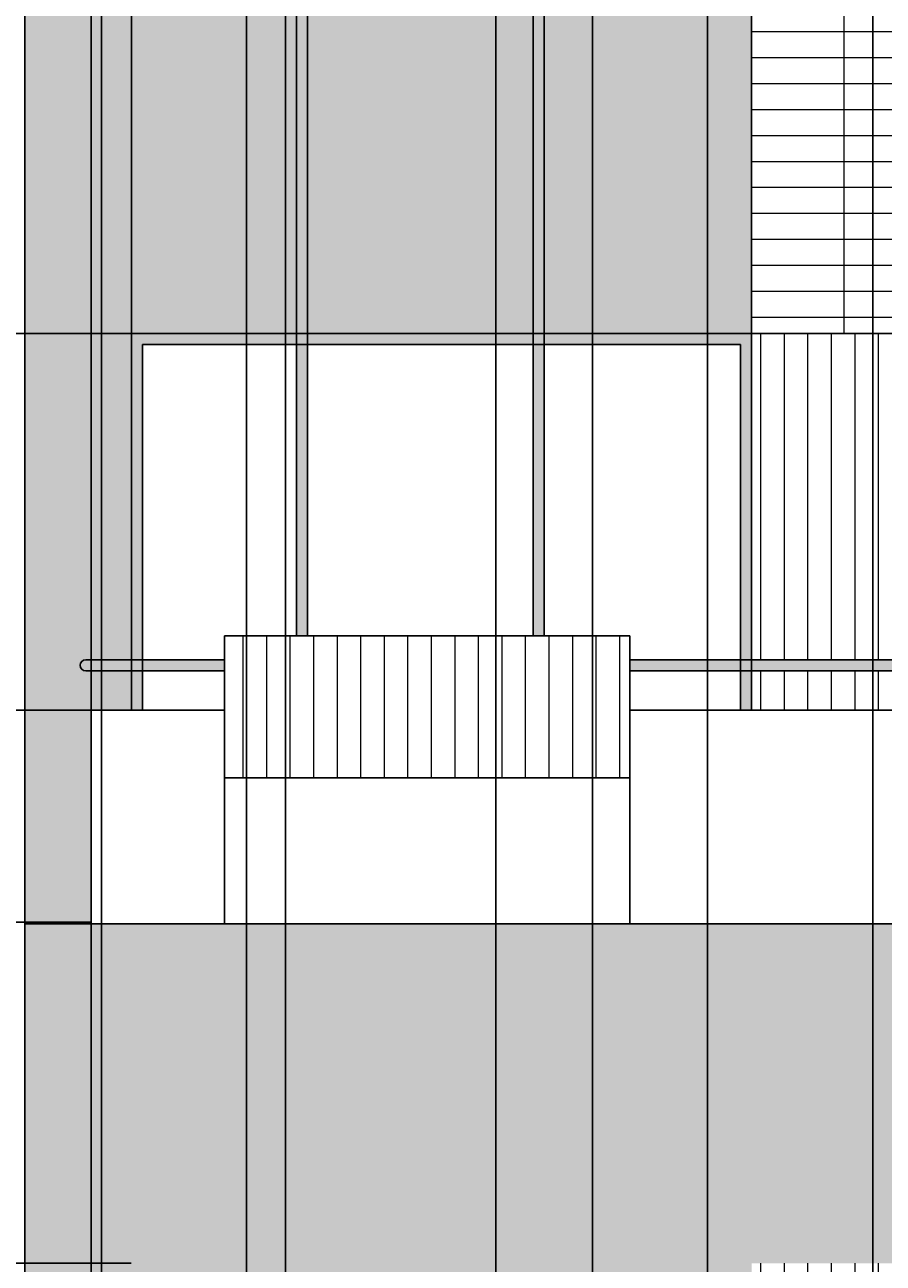
# Model space of a CAD drawing. Units: inches. Extents: x 241 to 943, y 109 to 1396.
# Tile 19 of 34: x 377 to 532, y 842 to 1065. Entities that reach past the tile are written whole.
import ezdxf

# ---------------------------------------------------------------- set-up
doc = ezdxf.new("R2010")
doc.units = ezdxf.units.IN
doc.header["$MEASUREMENT"] = 0
for name, color, linetype, lineweight in [('A-ANNO-DIMS', 2, 'Continuous', 18), ('A-ELEV', 7, 'Continuous', 25), ('A-ELEV-SHAD', 9, 'Continuous', 13), ('A-GLAZ-PATT', 18, 'Continuous', 13), ('A-WALL-PATT', 8, 'Continuous', 13)]:
    doc.layers.add(name, color=color, linetype=linetype, lineweight=lineweight)
doc.styles.get("Standard").update_dxf_attribs({"font": 'arial.ttf'})
doc.dimstyles.get("Standard").update_dxf_attribs({"dimtxt": 1.4375, "dimasz": 0.18, "dimexe": 0.18, "dimexo": 0.0625, "dimgap": 0.09, "dimtad": 0, "dimtih": 1, "dimtoh": 1, "dimdec": 4, "dimzin": 0, "dimdsep": 46, "dimlunit": 4, "dimtxsty": 'Standard', "dimcen": 0.09, "dimadec": 0, "dimazin": 0, "dimtfac": 1, "dimtdec": 4, "dimtofl": 0, "dimtmove": 0, "dimatfit": 3, "dimfxl": 1, "dimtolj": 1, "dimtzin": 0, "dimarcsym": 0})

# ---------------------------------------------------------------- blocks, each defined once
blk = doc.blocks.new('BALCONY-RAIL')
for p, q in [((26.08, 26.37), (26.08, 52.06)), ((26.08, 52.06), (99.3, 52.06)), ((99.3, 52.06), (99.3, 26.37)), ((3.52, 47.73), (1, 47.73)), ((3.52, 47.73), (26.08, 47.73)), ((3.52, 45.73), (1, 45.73)), ((3.52, 45.73), (26.08, 45.73)), ((99.3, 26.37), (26.08, 26.37)), ((26.08, 26.37), (26.08, 0)), ((99.3, 26.37), (99.3, 0))]:
    blk.add_line(p, q)
blk.add_arc((1, 46.73), 1, 90, 270)
blk = doc.blocks.new('*D7')
at = {"layer": 'A-ANNO-DIMS', "color": 0, "lineweight": -2, "transparency": 16777216}
for p, q in [((508.24, 1336.12), (244.31, 1336.12)), ((244.49, 1335.94), (244.49, 753.25)), ((244.49, 168.92), (244.49, 751.6)), ((303.17, 168.74), (244.31, 168.74))]:
    blk.add_line(p, q, dxfattribs=at)
at = {"layer": 'A-ANNO-DIMS', "color": 0, "transparency": 16777216}
for points in [[(244.46, 1335.94), (244.52, 1335.94), (244.49, 1336.12)], [(244.46, 168.92), (244.52, 168.92), (244.49, 168.74)]]:
    blk.add_solid(points, dxfattribs=at)
at = {"layer": 'Defpoints', "color": 0, "transparency": 16777216}
for p in [(244.49, 1336.12), (508.31, 1336.12), (303.24, 168.74)]:
    blk.add_point(p, dxfattribs=at)
at = {"layer": 'A-ANNO-DIMS', "color": 0, "transparency": 16777216, "insert": (244.49, 752.43), "char_height": 1.438, "attachment_point": 5}
blk.add_mtext('\\A1;1167.4', dxfattribs=at)
blk = doc.blocks.new('*D8')
at = {"layer": 'A-ANNO-DIMS', "color": 0, "lineweight": -2, "transparency": 16777216}
for p, q in [((377.04, 396.94), (377.04, 1395.05)), ((377.22, 1394.87), (380.96, 1394.87)), ((390.71, 1394.87), (386.97, 1394.87)), ((390.89, 384.24), (390.89, 1395.05))]:
    blk.add_line(p, q, dxfattribs=at)
at = {"layer": 'A-ANNO-DIMS', "color": 0, "transparency": 16777216}
for points in [[(377.22, 1394.9), (377.22, 1394.84), (377.04, 1394.87)], [(390.71, 1394.9), (390.71, 1394.84), (390.89, 1394.87)]]:
    blk.add_solid(points, dxfattribs=at)
at = {"layer": 'Defpoints', "color": 0, "transparency": 16777216}
for p in [(390.89, 1394.87), (377.04, 396.88), (390.89, 384.18)]:
    blk.add_point(p, dxfattribs=at)
at = {"layer": 'A-ANNO-DIMS', "color": 0, "transparency": 16777216, "insert": (383.97, 1394.87), "char_height": 1.438, "attachment_point": 5}
blk.add_mtext('\\A1;13.856', dxfattribs=at)
blk = doc.blocks.new('*D9')
at = {"layer": 'A-ANNO-DIMS', "color": 0, "lineweight": -2, "transparency": 16777216}
for p, q in [((390.89, 384.24), (390.89, 1395.05)), ((391.07, 1394.87), (424.13, 1394.87)), ((461.93, 1394.87), (428.87, 1394.87)), ((462.11, 384.24), (462.11, 1395.05))]:
    blk.add_line(p, q, dxfattribs=at)
at = {"layer": 'A-ANNO-DIMS', "color": 0, "transparency": 16777216}
for points in [[(391.07, 1394.9), (391.07, 1394.84), (390.89, 1394.87)], [(461.93, 1394.9), (461.93, 1394.84), (462.11, 1394.87)]]:
    blk.add_solid(points, dxfattribs=at)
at = {"layer": 'Defpoints', "color": 0, "transparency": 16777216}
for p in [(462.11, 1394.87), (390.89, 384.18), (462.11, 384.18)]:
    blk.add_point(p, dxfattribs=at)
at = {"layer": 'A-ANNO-DIMS', "color": 0, "transparency": 16777216, "insert": (426.5, 1394.87), "char_height": 1.438, "attachment_point": 5}
blk.add_mtext('\\A1;71.21', dxfattribs=at)
blk = doc.blocks.new('*D10')
at = {"layer": 'A-ANNO-DIMS', "color": 0, "lineweight": -2, "transparency": 16777216}
for p, q in [((462.11, 384.24), (462.11, 1395.05)), ((462.29, 1394.87), (468.4, 1394.87)), ((479.42, 1394.87), (473.3, 1394.87)), ((479.6, 384.24), (479.6, 1395.05))]:
    blk.add_line(p, q, dxfattribs=at)
at = {"layer": 'A-ANNO-DIMS', "color": 0, "transparency": 16777216}
for points in [[(462.29, 1394.9), (462.29, 1394.84), (462.11, 1394.87)], [(479.42, 1394.9), (479.42, 1394.84), (479.6, 1394.87)]]:
    blk.add_solid(points, dxfattribs=at)
at = {"layer": 'Defpoints', "color": 0, "transparency": 16777216}
for p in [(479.6, 1394.87), (462.11, 384.18), (479.6, 384.18)]:
    blk.add_point(p, dxfattribs=at)
at = {"layer": 'A-ANNO-DIMS', "color": 0, "transparency": 16777216, "insert": (470.85, 1394.87), "char_height": 1.438, "attachment_point": 5}
blk.add_mtext('\\A1;17.49', dxfattribs=at)
blk = doc.blocks.new('*D11')
at = {"layer": 'A-ANNO-DIMS', "color": 0, "lineweight": -2, "transparency": 16777216}
for p, q in [((500.33, 384.24), (500.33, 1395.05)), ((500.51, 1394.87), (513.31, 1394.87)), ((530.05, 1394.87), (517.25, 1394.87)), ((530.23, 384.24), (530.23, 1395.05))]:
    blk.add_line(p, q, dxfattribs=at)
at = {"layer": 'A-ANNO-DIMS', "color": 0, "transparency": 16777216}
for points in [[(500.51, 1394.9), (500.51, 1394.84), (500.33, 1394.87)], [(530.05, 1394.9), (530.05, 1394.84), (530.23, 1394.87)]]:
    blk.add_solid(points, dxfattribs=at)
at = {"layer": 'Defpoints', "color": 0, "transparency": 16777216}
for p in [(530.23, 1394.87), (500.33, 384.18), (530.23, 384.18)]:
    blk.add_point(p, dxfattribs=at)
at = {"layer": 'A-ANNO-DIMS', "color": 0, "transparency": 16777216, "insert": (515.28, 1394.87), "char_height": 1.438, "attachment_point": 5}
blk.add_mtext('\\A1;29.9', dxfattribs=at)
blk = doc.blocks.new('*D12')
at = {"layer": 'A-ANNO-DIMS', "color": 0, "lineweight": -2, "transparency": 16777216}
for p, q in [((530.23, 384.24), (530.23, 1395.05)), ((530.41, 1394.87), (587.56, 1394.87)), ((650.73, 1394.87), (593.58, 1394.87)), ((650.91, 384.24), (650.91, 1395.05))]:
    blk.add_line(p, q, dxfattribs=at)
at = {"layer": 'A-ANNO-DIMS', "color": 0, "transparency": 16777216}
for points in [[(530.41, 1394.9), (530.41, 1394.84), (530.23, 1394.87)], [(650.73, 1394.9), (650.73, 1394.84), (650.91, 1394.87)]]:
    blk.add_solid(points, dxfattribs=at)
at = {"layer": 'Defpoints', "color": 0, "transparency": 16777216}
for p in [(650.91, 1394.87), (530.23, 384.18), (650.91, 384.18)]:
    blk.add_point(p, dxfattribs=at)
at = {"layer": 'A-ANNO-DIMS', "color": 0, "transparency": 16777216, "insert": (590.57, 1394.87), "char_height": 1.438, "attachment_point": 5}
blk.add_mtext('\\A1;120.68', dxfattribs=at)
blk = doc.blocks.new('*D36')
at = {"layer": 'A-ANNO-DIMS', "color": 0, "lineweight": -2, "transparency": 16777216}
for p, q in [((396.25, 841.54), (244.31, 841.54)), ((244.49, 841.36), (244.49, 808.34)), ((244.49, 773.67), (244.49, 806.69)), ((396.25, 773.49), (244.31, 773.49))]:
    blk.add_line(p, q, dxfattribs=at)
at = {"layer": 'A-ANNO-DIMS', "color": 0, "transparency": 16777216}
for points in [[(244.46, 841.36), (244.52, 841.36), (244.49, 841.54)], [(244.46, 773.67), (244.52, 773.67), (244.49, 773.49)]]:
    blk.add_solid(points, dxfattribs=at)
at = {"layer": 'Defpoints', "color": 0, "transparency": 16777216}
for p in [(244.49, 841.54), (396.31, 841.54), (396.31, 773.49)]:
    blk.add_point(p, dxfattribs=at)
at = {"layer": 'A-ANNO-DIMS', "color": 0, "transparency": 16777216, "insert": (244.49, 807.51), "char_height": 1.438, "attachment_point": 5}
blk.add_mtext('\\A1;68.05', dxfattribs=at)
blk = doc.blocks.new('*D37')
at = {"layer": 'A-ANNO-DIMS', "color": 0, "lineweight": -2, "transparency": 16777216}
for p, q in [((388.98, 941.49), (244.31, 941.49)), ((244.49, 941.31), (244.49, 923.16)), ((244.49, 903.37), (244.49, 921.52)), ((388.98, 903.19), (244.31, 903.19))]:
    blk.add_line(p, q, dxfattribs=at)
at = {"layer": 'A-ANNO-DIMS', "color": 0, "transparency": 16777216}
for points in [[(244.46, 941.31), (244.52, 941.31), (244.49, 941.49)], [(244.46, 903.37), (244.52, 903.37), (244.49, 903.19)]]:
    blk.add_solid(points, dxfattribs=at)
at = {"layer": 'Defpoints', "color": 0, "transparency": 16777216}
for p in [(244.49, 941.49), (389.04, 941.49), (389.04, 903.19)]:
    blk.add_point(p, dxfattribs=at)
at = {"layer": 'A-ANNO-DIMS', "color": 0, "transparency": 16777216, "insert": (244.49, 922.34), "char_height": 1.438, "attachment_point": 5}
blk.add_mtext('\\A1;38.3', dxfattribs=at)
blk = doc.blocks.new('*D38')
at = {"layer": 'A-ANNO-DIMS', "color": 0, "lineweight": -2, "transparency": 16777216}
for p, q in [((396.25, 1009.54), (244.31, 1009.54)), ((244.49, 1009.36), (244.49, 976.34)), ((244.49, 941.67), (244.49, 974.69)), ((396.25, 941.49), (244.31, 941.49))]:
    blk.add_line(p, q, dxfattribs=at)
at = {"layer": 'A-ANNO-DIMS', "color": 0, "transparency": 16777216}
for points in [[(244.46, 1009.36), (244.52, 1009.36), (244.49, 1009.54)], [(244.46, 941.67), (244.52, 941.67), (244.49, 941.49)]]:
    blk.add_solid(points, dxfattribs=at)
at = {"layer": 'Defpoints', "color": 0, "transparency": 16777216}
for p in [(244.49, 1009.54), (396.31, 1009.54), (396.31, 941.49)]:
    blk.add_point(p, dxfattribs=at)
at = {"layer": 'A-ANNO-DIMS', "color": 0, "transparency": 16777216, "insert": (244.49, 975.51), "char_height": 1.438, "attachment_point": 5}
blk.add_mtext('\\A1;68.05', dxfattribs=at)
blk = doc.blocks.new('*D61')
at = {"layer": 'A-ANNO-DIMS', "color": 0, "lineweight": -2, "transparency": 16777216}
for p, q in [((377.04, 400.89), (377.04, 1395.05)), ((377.22, 1394.87), (398.03, 1394.87)), ((423.93, 1394.87), (403.12, 1394.87)), ((424.11, 568.89), (424.11, 1395.05))]:
    blk.add_line(p, q, dxfattribs=at)
at = {"layer": 'A-ANNO-DIMS', "color": 0, "transparency": 16777216}
for points in [[(377.22, 1394.9), (377.22, 1394.84), (377.04, 1394.87)], [(423.93, 1394.9), (423.93, 1394.84), (424.11, 1394.87)]]:
    blk.add_solid(points, dxfattribs=at)
at = {"layer": 'Defpoints', "color": 0, "transparency": 16777216}
for p in [(424.11, 1394.87), (424.11, 568.83), (377.04, 400.83)]:
    blk.add_point(p, dxfattribs=at)
at = {"layer": 'A-ANNO-DIMS', "color": 0, "transparency": 16777216, "insert": (400.57, 1394.87), "char_height": 1.438, "attachment_point": 5}
blk.add_mtext('\\A1;47.07', dxfattribs=at)
blk = doc.blocks.new('*D62')
at = {"layer": 'A-ANNO-DIMS', "color": 0, "lineweight": -2, "transparency": 16777216}
for p, q in [((424.11, 568.89), (424.11, 1395.05)), ((424.29, 1394.87), (492.35, 1394.87)), ((565.02, 1394.87), (496.96, 1394.87)), ((565.2, 568.89), (565.2, 1395.05))]:
    blk.add_line(p, q, dxfattribs=at)
at = {"layer": 'A-ANNO-DIMS', "color": 0, "transparency": 16777216}
for points in [[(424.29, 1394.9), (424.29, 1394.84), (424.11, 1394.87)], [(565.02, 1394.9), (565.02, 1394.84), (565.2, 1394.87)]]:
    blk.add_solid(points, dxfattribs=at)
at = {"layer": 'Defpoints', "color": 0, "transparency": 16777216}
for p in [(565.2, 1394.87), (424.11, 568.83), (565.2, 568.83)]:
    blk.add_point(p, dxfattribs=at)
at = {"layer": 'A-ANNO-DIMS', "color": 0, "transparency": 16777216, "insert": (494.66, 1394.87), "char_height": 1.438, "attachment_point": 5}
blk.add_mtext('\\A1;141.1', dxfattribs=at)
blk = doc.blocks.new('*D65')
at = {"layer": 'A-ANNO-DIMS', "color": 0, "lineweight": -2, "transparency": 16777216}
for p, q in [((424.11, 700.85), (424.11, 1395.05)), ((424.29, 1394.87), (505.52, 1394.87)), ((592.77, 1394.87), (511.54, 1394.87)), ((592.95, 700.85), (592.95, 1395.05))]:
    blk.add_line(p, q, dxfattribs=at)
at = {"layer": 'A-ANNO-DIMS', "color": 0, "transparency": 16777216}
for points in [[(424.29, 1394.9), (424.29, 1394.84), (424.11, 1394.87)], [(592.77, 1394.9), (592.77, 1394.84), (592.95, 1394.87)]]:
    blk.add_solid(points, dxfattribs=at)
at = {"layer": 'Defpoints', "color": 0, "transparency": 16777216}
for p in [(592.95, 1394.87), (424.11, 700.79), (592.95, 700.79)]:
    blk.add_point(p, dxfattribs=at)
at = {"layer": 'A-ANNO-DIMS', "color": 0, "transparency": 16777216, "insert": (508.53, 1394.87), "char_height": 1.438, "attachment_point": 5}
blk.add_mtext('\\A1;168.85', dxfattribs=at)
blk = doc.blocks.new('*D67')
at = {"layer": 'A-ANNO-DIMS', "color": 0, "lineweight": -2, "transparency": 16777216}
for p, q in [((389.04, 773.55), (389.04, 1395.05)), ((389.22, 1394.87), (495.34, 1394.87)), ((607.64, 1394.87), (501.52, 1394.87)), ((607.82, 773.55), (607.82, 1395.05))]:
    blk.add_line(p, q, dxfattribs=at)
at = {"layer": 'A-ANNO-DIMS', "color": 0, "transparency": 16777216}
for points in [[(389.22, 1394.9), (389.22, 1394.84), (389.04, 1394.87)], [(607.64, 1394.9), (607.64, 1394.84), (607.82, 1394.87)]]:
    blk.add_solid(points, dxfattribs=at)
at = {"layer": 'Defpoints', "color": 0, "transparency": 16777216}
for p in [(607.82, 1394.87), (389.04, 773.49), (607.82, 773.49)]:
    blk.add_point(p, dxfattribs=at)
at = {"layer": 'A-ANNO-DIMS', "color": 0, "transparency": 16777216, "insert": (498.43, 1394.87), "char_height": 1.438, "attachment_point": 5}
blk.add_mtext('\\A1;218.77', dxfattribs=at)
blk = doc.blocks.new('*D69')
at = {"layer": 'A-ANNO-DIMS', "color": 0, "lineweight": -2, "transparency": 16777216}
for p, q in [((389.04, 941.55), (389.04, 1395.05)), ((389.22, 1394.87), (476.28, 1394.87)), ((567.95, 1394.87), (480.9, 1394.87)), ((568.13, 941.55), (568.13, 1395.05))]:
    blk.add_line(p, q, dxfattribs=at)
at = {"layer": 'A-ANNO-DIMS', "color": 0, "transparency": 16777216}
for points in [[(389.22, 1394.9), (389.22, 1394.84), (389.04, 1394.87)], [(567.95, 1394.9), (567.95, 1394.84), (568.13, 1394.87)]]:
    blk.add_solid(points, dxfattribs=at)
at = {"layer": 'Defpoints', "color": 0, "transparency": 16777216}
for p in [(568.13, 1394.87), (389.04, 941.49), (568.13, 941.49)]:
    blk.add_point(p, dxfattribs=at)
at = {"layer": 'A-ANNO-DIMS', "color": 0, "transparency": 16777216, "insert": (478.59, 1394.87), "char_height": 1.438, "attachment_point": 5}
blk.add_mtext('\\A1;179.1', dxfattribs=at)
blk = doc.blocks.new('*D79')
at = {"layer": 'A-ANNO-DIMS', "color": 0, "lineweight": -2, "transparency": 16777216}
for p, q in [((479.6, 384.24), (479.6, 1395.05)), ((479.78, 1394.87), (486.88, 1394.87)), ((500.15, 1394.87), (493.05, 1394.87)), ((500.33, 384.24), (500.33, 1395.05))]:
    blk.add_line(p, q, dxfattribs=at)
at = {"layer": 'A-ANNO-DIMS', "color": 0, "transparency": 16777216}
for points in [[(479.78, 1394.9), (479.78, 1394.84), (479.6, 1394.87)], [(500.15, 1394.9), (500.15, 1394.84), (500.33, 1394.87)]]:
    blk.add_solid(points, dxfattribs=at)
at = {"layer": 'Defpoints', "color": 0, "transparency": 16777216}
for p in [(500.33, 1394.87), (479.6, 384.18), (500.33, 384.18)]:
    blk.add_point(p, dxfattribs=at)
at = {"layer": 'A-ANNO-DIMS', "color": 0, "transparency": 16777216, "insert": (489.96, 1394.87), "char_height": 1.438, "attachment_point": 5}
blk.add_mtext('\\A1;20.736', dxfattribs=at)
blk = doc.blocks.new('*D89')
at = {"layer": 'A-ANNO-DIMS', "color": 0, "lineweight": -2, "transparency": 16777216}
for p, q in [((377.04, 841.6), (377.04, 1395.05)), ((377.22, 1394.87), (494.32, 1394.87)), ((617.58, 1394.87), (500.48, 1394.87)), ((617.76, 841.6), (617.76, 1395.05))]:
    blk.add_line(p, q, dxfattribs=at)
at = {"layer": 'A-ANNO-DIMS', "color": 0, "transparency": 16777216}
for points in [[(377.22, 1394.9), (377.22, 1394.84), (377.04, 1394.87)], [(617.58, 1394.9), (617.58, 1394.84), (617.76, 1394.87)]]:
    blk.add_solid(points, dxfattribs=at)
at = {"layer": 'Defpoints', "color": 0, "transparency": 16777216}
for p in [(617.76, 1394.87), (377.04, 841.54), (617.76, 841.54)]:
    blk.add_point(p, dxfattribs=at)
at = {"layer": 'A-ANNO-DIMS', "color": 0, "transparency": 16777216, "insert": (497.4, 1394.87), "char_height": 1.438, "attachment_point": 5}
blk.add_mtext('\\A1;240.72', dxfattribs=at)
blk = doc.blocks.new('*D91')
at = {"layer": 'A-ANNO-DIMS', "color": 0, "lineweight": -2, "transparency": 16777216}
for p, q in [((377.04, 1070.79), (377.04, 109.81)), ((389.04, 1070.79), (389.04, 109.81)), ((377.22, 109.99), (380.04, 109.99)), ((388.86, 109.99), (386.04, 109.99))]:
    blk.add_line(p, q, dxfattribs=at)
at = {"layer": 'A-ANNO-DIMS', "color": 0, "transparency": 16777216}
for points in [[(377.22, 110.02), (377.22, 109.96), (377.04, 109.99)], [(388.86, 110.02), (388.86, 109.96), (389.04, 109.99)]]:
    blk.add_solid(points, dxfattribs=at)
at = {"layer": 'Defpoints', "color": 0, "transparency": 16777216}
for p in [(377.04, 1070.85), (389.04, 1070.85), (389.04, 109.99)]:
    blk.add_point(p, dxfattribs=at)
at = {"layer": 'A-ANNO-DIMS', "color": 0, "transparency": 16777216, "insert": (383.04, 109.99), "char_height": 1.438, "attachment_point": 5}
blk.add_mtext('\\A1;12.004', dxfattribs=at)
blk = doc.blocks.new('*D99')
at = {"layer": 'A-ANNO-DIMS', "color": 0, "lineweight": -2, "transparency": 16777216}
for p, q in [((417.09, 181.71), (417.09, 1395.05)), ((417.27, 1394.87), (539.16, 1394.87)), ((667.21, 1394.87), (545.33, 1394.87)), ((667.39, 214.58), (667.39, 1395.05))]:
    blk.add_line(p, q, dxfattribs=at)
at = {"layer": 'A-ANNO-DIMS', "color": 0, "transparency": 16777216}
for points in [[(417.27, 1394.9), (417.27, 1394.84), (417.09, 1394.87)], [(667.21, 1394.9), (667.21, 1394.84), (667.39, 1394.87)]]:
    blk.add_solid(points, dxfattribs=at)
at = {"layer": 'Defpoints', "color": 0, "transparency": 16777216}
for p in [(667.39, 1394.87), (667.39, 214.52), (417.09, 181.65)]:
    blk.add_point(p, dxfattribs=at)
at = {"layer": 'A-ANNO-DIMS', "color": 0, "transparency": 16777216, "insert": (542.24, 1394.87), "char_height": 1.438, "attachment_point": 5}
blk.add_mtext('\\A1;250.30', dxfattribs=at)
blk = doc.blocks.new('*D101')
at = {"layer": 'A-ANNO-DIMS', "color": 0, "lineweight": -2, "transparency": 16777216}
for p, q in [((396.31, 1009.6), (396.31, 1395.05)), ((396.49, 1394.87), (408.12, 1394.87)), ((425.94, 1394.87), (414.31, 1394.87)), ((426.12, 1007.6), (426.12, 1395.05))]:
    blk.add_line(p, q, dxfattribs=at)
at = {"layer": 'A-ANNO-DIMS', "color": 0, "transparency": 16777216}
for points in [[(396.49, 1394.9), (396.49, 1394.84), (396.31, 1394.87)], [(425.94, 1394.9), (425.94, 1394.84), (426.12, 1394.87)]]:
    blk.add_solid(points, dxfattribs=at)
at = {"layer": 'Defpoints', "color": 0, "transparency": 16777216}
for p in [(426.12, 1394.87), (396.31, 1009.54), (426.12, 1007.54)]:
    blk.add_point(p, dxfattribs=at)
at = {"layer": 'A-ANNO-DIMS', "color": 0, "transparency": 16777216, "insert": (411.21, 1394.87), "char_height": 1.438, "attachment_point": 5}
blk.add_mtext('\\A1;29.805', dxfattribs=at)
blk = doc.blocks.new('*D102')
at = {"layer": 'A-ANNO-DIMS', "color": 0, "lineweight": -2, "transparency": 16777216}
for p, q in [((428.12, 1007.6), (428.12, 1395.05)), ((428.3, 1394.87), (445.94, 1394.87)), ((468.69, 1394.87), (451.04, 1394.87)), ((468.87, 1007.6), (468.87, 1395.05))]:
    blk.add_line(p, q, dxfattribs=at)
at = {"layer": 'A-ANNO-DIMS', "color": 0, "transparency": 16777216}
for points in [[(428.3, 1394.9), (428.3, 1394.84), (428.12, 1394.87)], [(468.69, 1394.9), (468.69, 1394.84), (468.87, 1394.87)]]:
    blk.add_solid(points, dxfattribs=at)
at = {"layer": 'Defpoints', "color": 0, "transparency": 16777216}
for p in [(468.87, 1394.87), (428.12, 1007.54), (468.87, 1007.54)]:
    blk.add_point(p, dxfattribs=at)
at = {"layer": 'A-ANNO-DIMS', "color": 0, "transparency": 16777216, "insert": (448.49, 1394.87), "char_height": 1.438, "attachment_point": 5}
blk.add_mtext('\\A1;40.75', dxfattribs=at)
blk = doc.blocks.new('*D103')
at = {"layer": 'A-ANNO-DIMS', "color": 0, "lineweight": -2, "transparency": 16777216}
for p, q in [((470.87, 1007.6), (470.87, 1395.05)), ((471.05, 1394.87), (487.08, 1394.87)), ((508.13, 1394.87), (492.1, 1394.87)), ((508.31, 1009.6), (508.31, 1395.05))]:
    blk.add_line(p, q, dxfattribs=at)
at = {"layer": 'A-ANNO-DIMS', "color": 0, "transparency": 16777216}
for points in [[(471.05, 1394.9), (471.05, 1394.84), (470.87, 1394.87)], [(508.13, 1394.9), (508.13, 1394.84), (508.31, 1394.87)]]:
    blk.add_solid(points, dxfattribs=at)
at = {"layer": 'Defpoints', "color": 0, "transparency": 16777216}
for p in [(508.31, 1394.87), (508.31, 1009.54), (470.87, 1007.54)]:
    blk.add_point(p, dxfattribs=at)
at = {"layer": 'A-ANNO-DIMS', "color": 0, "transparency": 16777216, "insert": (489.59, 1394.87), "char_height": 1.438, "attachment_point": 5}
blk.add_mtext('\\A1;37.44', dxfattribs=at)

msp = doc.modelspace()

# ---------------------------------------------------------------- hatches: boundary and pattern name
at = {"layer": 'A-ELEV-SHAD'}
h = msp.add_hatch(color=256, dxfattribs=at)
h.dxf.hatch_style = 1
h.paths.add_polyline_path([(508.3064, 1070.8538), (377.0391, 1070.8538), (377.0391, 1009.5382), (508.3064, 1009.5382)])
h.paths.add_polyline_path([(508.3064, 1238.8538), (377.0391, 1238.8538), (377.0391, 1177.5382), (508.3064, 1177.5382)])
h.paths.add_polyline_path([(581.3632, 902.8538), (568.1348, 902.8538), (553.5166, 902.8538), (377.0391, 902.8538), (377.0391, 841.5382), (553.5166, 841.5382), (564.8076, 841.5382), (581.3632, 841.5382)])
h.paths.add_polyline_path([(820.8374, 1275.9142), (747.7579, 1275.9142), (747.7579, 1238.8538), (820.8374, 1238.8538)])
h.paths.add_polyline_path([(820.8374, 1238.8538), (747.7579, 1238.8538), (747.9341, 1223.0633), (820.8374, 1223.0633)])
h.paths.add_polyline_path([(396.3125, 841.5382), (377.0391, 841.5382), (377.0391, 734.8538), (389.0429, 734.8538), (389.0429, 735.188), (389.0429, 773.4916), (396.3125, 773.4916), (396.3125, 780.5808), (390.5597, 780.5808), (388.0428, 780.5808, -1), (388.0428, 782.5808), (390.5597, 782.5808), (396.3125, 782.5808)])
h = msp.add_hatch(color=256, dxfattribs=at)
h.dxf.hatch_style = 1
h.paths.add_polyline_path([(537.4269, 698.7912), (534.1778, 698.7912), (534.1778, 659.3434), (537.4269, 659.3434)])
h.paths.add_polyline_path([(508.0803, 698.7912), (450.9259, 698.7912), (450.9259, 659.3434), (452.9259, 659.3434), (452.9259, 696.7912), (506.0803, 696.7912), (506.0803, 659.3434), (508.0803, 659.3434)])
h.paths.add_polyline_path([(481.5031, 696.7912), (479.5031, 696.7912), (479.5031, 659.3434), (481.5031, 659.3434)], flags=17)
h.paths.add_polyline_path([(481.5031, 657.3434), (479.5031, 657.3434), (479.5031, 653.3371), (481.5031, 653.3371)], flags=17)
h.paths.add_polyline_path([(508.0803, 657.3434), (506.0803, 657.3434), (506.0803, 653.3371), (452.9259, 653.3371), (452.9259, 657.3434), (450.9259, 657.3434), (450.9259, 651.3371), (508.0803, 651.3371)])
h.paths.add_polyline_path([(428.1173, 839.5382), (426.1173, 839.5382), (426.1173, 786.9154), (428.1173, 786.9154)], flags=17)
h.paths.add_polyline_path([(470.8692, 839.5382), (468.8692, 839.5382), (468.8692, 786.9154), (470.8692, 786.9154)], flags=17)
h.paths.add_polyline_path([(508.3064, 841.5382), (396.3125, 841.5382), (396.3125, 782.5808), (398.3125, 782.5808), (398.3125, 839.5382), (506.3064, 839.5382), (506.3064, 782.5808), (508.3064, 782.5808)])
h.paths.add_polyline_path([(398.3125, 780.5808), (396.3125, 780.5808), (396.3125, 773.4916), (398.3125, 773.4916)])
h.paths.add_polyline_path([(508.3064, 780.5808), (506.3064, 780.5808), (506.3064, 773.4916), (508.3064, 773.4916)])
h.paths.add_polyline_path([(715.6236, 841.5382), (678.2674, 841.5382), (678.2674, 734.8538), (715.6236, 734.8538)])
h.paths.add_polyline_path([(680.2674, 839.5382), (682.4526, 839.5382), (713.6236, 839.5382), (713.6236, 736.9235), (690.2047, 736.9235), (680.2674, 736.9235)], flags=16)
h.paths.add_polyline_path([(792.691, 841.5382), (747.7579, 841.5382), (747.7579, 734.8538), (754.5373, 734.8538), (754.5373, 736.9235), (754.5373, 839.5382), (756.7224, 839.5382), (787.8934, 839.5382), (787.8934, 765.9585), (792.691, 765.9585)])
h.paths.add_polyline_path([(659.2925, 1009.5382), (657.2925, 1009.5382), (657.2925, 902.8538), (659.2925, 902.8538)])
h.paths.add_polyline_path([(751.5078, 976.6275), (712.5839, 976.6275), (712.5839, 974.6275), (751.5078, 974.6275)])
h.paths.add_polyline_path([(470.8692, 1007.5382), (468.8692, 1007.5382), (468.8692, 954.9154), (470.8692, 954.9154)], flags=17)
h.paths.add_polyline_path([(508.3064, 1009.5382), (396.3125, 1009.5382), (396.3125, 950.5808), (398.3125, 950.5808), (398.3125, 1007.5382), (506.3064, 1007.5382), (506.3064, 950.5808), (508.3064, 950.5808)])
h.paths.add_polyline_path([(428.1173, 1007.5382), (426.1173, 1007.5382), (426.1173, 954.9154), (428.1173, 954.9154)], flags=17)
h.paths.add_polyline_path([(398.3125, 948.5808), (396.3125, 948.5808), (396.3125, 941.4916), (398.3125, 941.4916)])
h.paths.add_polyline_path([(508.3064, 948.5808), (506.3064, 948.5808), (506.3064, 941.4916), (508.3064, 941.4916)])
h.paths.add_polyline_path([(428.1173, 1175.5382), (426.1173, 1175.5382), (426.1173, 1122.9154), (428.1173, 1122.9154)], flags=17)
h.paths.add_polyline_path([(508.3064, 1177.5382), (396.3125, 1177.5382), (396.3125, 1118.5808), (398.3125, 1118.5808), (398.3125, 1175.5382), (506.3064, 1175.5382), (506.3064, 1118.5808), (506.8039, 1118.5808, -1), (506.8039, 1116.5808), (506.3064, 1116.5808), (506.3064, 1109.4916), (508.3064, 1109.4916)])
h.paths.add_polyline_path([(470.8692, 1175.5382), (468.8692, 1175.5382), (468.8692, 1122.9154), (470.8692, 1122.9154)], flags=17)
h.paths.add_polyline_path([(398.3125, 1116.5808), (396.3125, 1116.5808), (396.3125, 1109.4916), (398.3125, 1109.4916)], flags=17)
h.paths.add_polyline_path([(724.819, 1177.7336), (533.952, 1177.7336), (533.952, 1108.1686), (724.819, 1108.1686)])
h.paths.add_polyline_path([(535.952, 1175.7336), (722.819, 1175.7336), (722.819, 1110.1686), (535.952, 1110.1686)], flags=0)
h.paths.add_polyline_path([(622.521, 1136.0739), (643.4534, 1136.0739), (643.4534, 1134.0739), (622.521, 1134.0739)], flags=0)
h.paths.add_polyline_path([(722.819, 1175.7336), (535.952, 1175.7336), (535.952, 1110.1686), (722.819, 1110.1686)], flags=16)
h.paths.add_polyline_path([(565.947, 1151.5772), (535.952, 1151.5772), (535.952, 1149.5772), (565.947, 1149.5772)], flags=0)
h = msp.add_hatch(color=256, dxfattribs=at)
h.dxf.hatch_style = 1
h.paths.add_polyline_path([(396.3125, 1009.5382), (377.0391, 1009.5382), (377.0391, 902.8538), (389.0429, 902.8538), (389.0429, 941.4916), (396.3125, 941.4916), (396.3125, 948.5808), (390.5597, 948.5808), (388.0428, 948.5808, -1), (388.0428, 950.5808), (390.5597, 950.5808), (396.3125, 950.5808)])
at = {"layer": 'A-GLAZ-PATT'}
h = msp.add_hatch(dxfattribs=at)
h.set_pattern_fill('ANSI31', color=256, scale=34, angle=45)
h.paths.add_polyline_path([(486.3418, 786.9154), (413.1187, 786.9154), (413.1187, 761.2284), (486.3418, 761.2284)])
h.paths.add_polyline_path([(486.3418, 954.9154), (413.1187, 954.9154), (413.1187, 929.2284), (486.3418, 929.2284)])
h.paths.add_polyline_path([(462.1074, 289.6933), (390.895, 289.6933), (390.895, 277.4626), (390.895, 274.3507), (462.1074, 274.3507), (462.1074, 277.4626)])
h.paths.add_polyline_path([(500.3323, 289.6933), (479.596, 289.6933), (479.596, 274.3507), (500.3323, 274.3507)])
h.paths.add_polyline_path([(450.9259, 566.8295), (426.1086, 566.8295), (426.1086, 498.4395), (446.4348, 498.4395), (446.4348, 519.3754), (450.9259, 519.3754), (450.9259, 525.3816), (445.5808, 525.3816, -1), (445.5808, 527.3816), (450.9259, 527.3816)])
h.paths.add_polyline_path([(563.2023, 508.9074), (534.1778, 508.9074), (508.1906, 508.9074), (508.1906, 498.4395), (563.2023, 498.4395)])
h.paths.add_polyline_path([(747.6328, 700.7912), (712.0171, 700.7912), (712.0171, 628.4013), (747.6328, 628.4013)])
h.paths.add_polyline_path([(446.4348, 643.7483), (426.1086, 643.7483), (426.1086, 630.4013), (446.4348, 630.4013)])
h.paths.add_polyline_path([(564.8076, 841.5382), (553.5166, 841.5382), (508.3064, 841.5382), (508.3064, 782.5808), (564.8076, 782.5808)])
h.paths.add_polyline_path([(564.8076, 780.5808), (508.3064, 780.5808), (508.3064, 773.4916), (564.8076, 773.4916)])
h.paths.add_polyline_path([(792.691, 762.5799), (759.6248, 762.5799), (759.6248, 736.9235), (759.6248, 734.8538), (792.691, 734.8538)])
h.paths.add_polyline_path([(564.8076, 1009.5382), (553.5166, 1009.5382), (508.3064, 1009.5382), (508.3064, 950.5808), (562.3033, 950.5808, -1), (562.3033, 948.5808), (508.3064, 948.5808), (508.3064, 941.4916), (564.8076, 941.4916)])
h.paths.add_polyline_path([(486.3418, 1122.9154), (413.1187, 1122.9154), (413.1187, 1097.2284), (486.3418, 1097.2284)])
h = msp.add_hatch(color=256, dxfattribs=at)
h.dxf.hatch_style = 1
h.paths.add_polyline_path([(396.3125, 1118.5808), (390.5597, 1118.5808), (388.0428, 1118.5808, 1), (388.0428, 1116.5808), (390.5597, 1116.5808), (396.3125, 1116.5808)])
h.paths.add_polyline_path([(398.3125, 1118.5808), (396.3125, 1118.5808), (396.3125, 1116.5808), (398.3125, 1116.5808)])
h.paths.add_polyline_path([(413.1187, 1118.5808), (398.3125, 1118.5808), (398.3125, 1116.5808), (413.1187, 1116.5808)])
h.paths.add_polyline_path([(506.3064, 1118.5808), (486.3418, 1118.5808), (486.3418, 1116.5808), (506.3064, 1116.5808)])
h.paths.add_polyline_path([(506.8039, 1118.5808), (506.3064, 1118.5808), (506.3064, 1116.5808), (506.8039, 1116.5808, 1)])
h.paths.add_polyline_path([(396.3125, 950.5808), (390.5597, 950.5808), (388.0428, 950.5808, 1), (388.0428, 948.5808), (390.5597, 948.5808), (396.3125, 948.5808)])
h.paths.add_polyline_path([(398.3125, 950.5808), (396.3125, 950.5808), (396.3125, 948.5808), (398.3125, 948.5808)])
h.paths.add_polyline_path([(413.1187, 950.5808), (398.3125, 950.5808), (398.3125, 948.5808), (413.1187, 948.5808)])
h.paths.add_polyline_path([(506.3064, 950.5808), (486.3418, 950.5808), (486.3418, 948.5808), (506.3064, 948.5808)])
h.paths.add_polyline_path([(508.3064, 950.5808), (506.3064, 950.5808), (506.3064, 948.5808), (508.3064, 948.5808)])
h.paths.add_polyline_path([(562.3033, 950.5808), (508.3064, 950.5808), (508.3064, 948.5808), (562.3033, 948.5808, 1)])
h.paths.add_polyline_path([(396.3125, 782.5808), (390.5597, 782.5808), (388.0428, 782.5808, 1), (388.0428, 780.5808), (390.5597, 780.5808), (396.3125, 780.5808)])
h.paths.add_polyline_path([(398.3125, 782.5808), (396.3125, 782.5808), (396.3125, 780.5808), (398.3125, 780.5808)])
h.paths.add_polyline_path([(413.1187, 782.5808), (398.3125, 782.5808), (398.3125, 780.5808), (413.1187, 780.5808)])
h.paths.add_polyline_path([(506.3064, 782.5808), (486.3418, 782.5808), (486.3418, 780.5808), (506.3064, 780.5808)])
h.paths.add_polyline_path([(508.3064, 782.5808), (506.3064, 782.5808), (506.3064, 780.5808), (508.3064, 780.5808)])
h.paths.add_polyline_path([(564.8076, 782.5808), (508.3064, 782.5808), (508.3064, 780.5808), (564.8076, 780.5808)])
h.paths.add_polyline_path([(605.9087, 782.5808), (564.8076, 782.5808), (564.8076, 780.5808), (605.9087, 780.5808, 1)])
h.paths.add_polyline_path([(450.9259, 659.3434), (445.5808, 659.3434, 1), (445.5808, 657.3434), (450.9259, 657.3434)])
h.paths.add_polyline_path([(452.9259, 659.3434), (450.9259, 659.3434), (450.9259, 657.3434), (452.9259, 657.3434)])
h.paths.add_polyline_path([(506.0803, 659.3434), (452.9259, 659.3434), (452.9259, 657.3434), (506.0803, 657.3434)])
h.paths.add_polyline_path([(508.0803, 659.3434), (506.0803, 659.3434), (506.0803, 657.3434), (508.0803, 657.3434)])
h.paths.add_polyline_path([(563.2023, 659.3434), (537.4269, 659.3434), (537.4269, 657.3434), (563.2023, 657.3434)])
h.paths.add_polyline_path([(590.8792, 659.3434), (563.9297, 659.3434), (563.9297, 657.3434), (590.8792, 657.3434)])
h.paths.add_polyline_path([(563.9297, 659.3434), (563.2023, 659.3434), (563.2023, 657.3434), (563.9297, 657.3434)])
h.paths.add_polyline_path([(537.4269, 659.3434), (534.1778, 659.3434), (534.1778, 657.3434), (537.4269, 657.3434)])
h.paths.add_polyline_path([(534.1778, 659.3434), (508.0803, 659.3434), (508.0803, 657.3434), (534.1778, 657.3434)])
h.paths.add_polyline_path([(450.9259, 527.3816), (445.5808, 527.3816, 1), (445.5808, 525.3816), (450.9259, 525.3816)])
h.paths.add_polyline_path([(452.9259, 527.3816), (450.9259, 527.3816), (450.9259, 525.3816), (452.9259, 525.3816)])
h.paths.add_polyline_path([(479.5031, 527.3816), (452.9259, 527.3816), (452.9259, 525.3816), (479.5031, 525.3816)])
h.paths.add_polyline_path([(481.5031, 527.3816), (479.5031, 527.3816), (479.5031, 525.3816), (481.5031, 525.3816)])
h.paths.add_polyline_path([(506.0803, 527.3816), (481.5031, 527.3816), (481.5031, 525.3816), (506.0803, 525.3816)])
h.paths.add_polyline_path([(508.0803, 527.3816), (506.0803, 527.3816), (506.0803, 525.3816), (508.0803, 525.3816)])
h.paths.add_polyline_path([(563.2023, 527.3816), (508.0803, 527.3816), (508.0803, 525.3816), (563.2023, 525.3816)])
at = {"layer": 'A-WALL-PATT'}
h = msp.add_hatch(dxfattribs=at)
h.set_pattern_fill('GRATE', color=256, scale=150)
h.paths.add_polyline_path([(747.7579, 1238.8538), (747.7579, 1275.9142), (747.7579, 1336.1154), (508.3064, 1336.1154), (508.3064, 1275.9142), (508.3064, 1238.8538), (508.3064, 1177.5382), (508.3064, 1109.4916), (508.3064, 1070.8538), (553.5166, 1070.8538), (749.6328, 1070.8538)])
h.paths.add_polyline_path([(533.952, 1108.1686), (533.952, 1177.7336), (533.952, 1303.0286), (724.819, 1303.0286), (724.819, 1108.1686)], flags=16)
h.paths.add_polyline_path([(535.952, 1110.1686), (535.952, 1175.7336), (722.819, 1175.7336), (722.819, 1110.1686)], flags=0)
h.paths.add_polyline_path([(643.4534, 1134.0739), (622.521, 1134.0739), (622.521, 1136.0739), (643.4534, 1136.0739)], flags=0)
h.paths.add_polyline_path([(617.7594, 568.8295), (617.7594, 734.8538), (377.0391, 734.8538), (377.0391, 566.8538), (377.0391, 400.8295), (417.0913, 400.8295), (618.9643, 400.8295)])
h.paths.add_polyline_path([(424.1086, 496.4395), (424.1086, 568.8295), (565.2023, 568.8295), (565.2023, 496.4395)], flags=16)
h.paths.add_polyline_path([(426.1086, 498.4395), (426.1086, 566.8295), (563.2023, 566.8295), (563.2023, 508.9074), (563.2023, 498.4395)], flags=0)
h.paths.add_polyline_path([(508.0803, 508.9074), (508.0803, 519.3754), (450.9259, 519.3754), (450.9259, 525.3816), (445.5808, 525.3816, -1), (445.5808, 527.3816), (450.9259, 527.3816), (450.9259, 566.8295), (508.0803, 566.8295), (537.4269, 566.8295), (537.4269, 508.9074)], flags=0)
h.paths.add_polyline_path([(506.0803, 521.3754), (452.9259, 521.3754), (452.9259, 564.8295), (506.0803, 564.8295)], flags=0)
h.paths.add_polyline_path([(424.1086, 628.4013), (424.1086, 700.7912), (592.9542, 700.7912), (592.9542, 628.4013)], flags=16)
h.paths.add_polyline_path([(426.1086, 630.4013), (426.1086, 698.7912), (590.8792, 698.7912), (590.8792, 630.4013)], flags=0)
h.paths.add_polyline_path([(508.1906, 651.3371), (508.0803, 651.3371), (450.9259, 651.3371), (428.0291, 651.3371), (428.0291, 698.7912), (451.9767, 698.7912), (508.0803, 698.7912), (537.4269, 698.7912), (563.2023, 698.7912), (563.2023, 659.3434), (563.9297, 659.3434), (563.9297, 651.3371)], flags=0)
h.paths.add_polyline_path([(506.0803, 653.3371), (452.9259, 653.3371), (452.9259, 657.3434), (445.5808, 657.3434, -1), (445.5808, 659.3434), (452.9259, 659.3434), (452.9259, 696.7912), (506.0803, 696.7912)], flags=0)
h = msp.add_hatch(dxfattribs=at)
h.set_pattern_fill('GRATE', color=256, scale=150)
h.paths.add_polyline_path([(820.8374, 1070.8538), (749.6328, 1070.8538), (553.5166, 1070.8538), (508.3064, 1070.8538), (508.3064, 1009.5382), (553.5166, 1009.5382), (564.8076, 1009.5382), (603.8694, 1009.5382), (751.5078, 1009.5382), (751.5078, 902.8538), (603.8694, 902.8538), (603.8694, 1009.5382), (564.8076, 1009.5382), (564.8076, 941.4916), (568.1348, 941.4916), (568.1348, 902.8538), (581.3632, 902.8538), (581.3632, 841.5382), (564.8076, 841.5382), (564.8076, 782.5808), (605.9087, 782.5808, -1), (605.9087, 780.5808), (564.8076, 780.5808), (564.8076, 773.4916), (597.514, 773.4916), (607.8162, 773.4916), (607.8162, 734.8538), (617.7594, 734.8538), (617.7594, 841.5382), (792.691, 841.5382), (792.691, 734.8538), (617.7594, 734.8538), (617.7594, 702.7912), (749.6328, 702.7912), (749.6328, 626.4013), (617.7594, 626.4013), (617.7594, 568.8295), (820.8374, 568.8295), (820.8374, 736.8295), (820.8374, 902.8538)])

# ---------------------------------------------------------------- linework, layer by layer
at = {"layer": 'A-ELEV'}
for p, q in [((377.0391, 902.8538), (377.0391, 1070.8538)), ((508.3064, 1009.5382), (508.3064, 1070.8538)), ((377.0391, 1009.5382), (553.5166, 1009.5382)), ((396.3125, 1009.5382), (396.3125, 941.4916)), ((508.3064, 1009.5382), (508.3064, 941.4916)), ((398.3125, 1007.5382), (506.3064, 1007.5382)), ((398.3125, 1007.5382), (398.3125, 941.4916)), ((426.1173, 1007.5382), (426.1173, 954.9154)), ((428.1173, 1007.5382), (428.1173, 954.9154)), ((468.8692, 1007.5382), (468.8692, 954.9154)), ((470.8692, 1007.5382), (470.8692, 954.9154)), ((506.3064, 1007.5382), (506.3064, 941.4916)), ((486.3418, 950.5808), (562.3033, 950.5808)), ((486.3418, 948.5808), (562.3033, 948.5808)), ((389.0429, 941.4916), (389.0429, 903.188)), ((389.0429, 941.4916), (413.1187, 941.4916)), ((568.1348, 941.4916), (486.3418, 941.4916)), ((377.0391, 734.8538), (377.0391, 902.8538)), ((553.5166, 902.8538), (377.0391, 902.8538))]:
    msp.add_line(p, q, dxfattribs=at)

# ---------------------------------------------------------------- block references
msp.add_blockref('BALCONY-RAIL', (387.043, 902.854), dxfattribs=at)

# ---------------------------------------------------------------- dimensions: what is measured, and where the dimension line sits
at = {"layer": 'A-ANNO-DIMS'}
for base, p1, p2, override, picture, middle in [((390.895, 1394.8654), (377.0391, 396.8782), (390.895, 384.1784), {"dimdec": 3, "dimlfac": 1, "dimrnd": 0, "dimzin": 0, "dimdsep": 46, "dimlunit": 2}, '*D8', (383.9671, 1394.8654)), ((424.1086, 1394.8654), (377.0391, 400.8295), (424.1086, 568.8295), {"dimdec": 2, "dimlfac": 1, "dimrnd": 0, "dimzin": 0, "dimdsep": 46, "dimlunit": 2}, '*D61', (400.5739, 1394.8654)), ((617.7594, 1394.8654), (377.0391, 841.5382), (617.7594, 841.5382), {"dimdec": 2, "dimlfac": 1, "dimrnd": 0, "dimzin": 0, "dimdsep": 46, "dimlunit": 2}, '*D89', (497.3993, 1394.8654)), ((607.8162, 1394.8654), (389.0429, 773.4916), (607.8162, 773.4916), {"dimdec": 2, "dimlfac": 1, "dimrnd": 0, "dimzin": 0, "dimdsep": 46, "dimlunit": 2}, '*D67', (498.4295, 1394.8654)), ((568.1348, 1394.8654), (389.0429, 941.4916), (568.1348, 941.4916), {"dimdec": 1, "dimlfac": 1, "dimrnd": 0, "dimzin": 0, "dimdsep": 46, "dimlunit": 2}, '*D69', (478.5888, 1394.8654)), ((462.1074, 1394.8654), (390.895, 384.1784), (462.1074, 384.1784), {"dimdec": 2, "dimlfac": 1, "dimrnd": 0, "dimzin": 0, "dimdsep": 46, "dimlunit": 2}, '*D9', (426.5012, 1394.8654)), ((426.1173, 1394.8654), (396.3125, 1009.5382), (426.1173, 1007.5382), {"dimdec": 3, "dimlfac": 1, "dimrnd": 0, "dimzin": 0, "dimdsep": 46, "dimlunit": 2}, '*D101', (411.2149, 1394.8654)), ((667.3935, 1394.8654), (417.0913, 181.649), (667.3935, 214.5189), {"dimdec": 2, "dimlfac": 1, "dimrnd": 0, "dimzin": 0, "dimdsep": 46, "dimlunit": 2}, '*D99', (542.2424, 1394.8654)), ((565.2023, 1394.8654), (424.1086, 568.8295), (565.2023, 568.8295), {"dimdec": 1, "dimlfac": 1, "dimrnd": 0, "dimzin": 0, "dimdsep": 46, "dimlunit": 2}, '*D62', (494.6554, 1394.8654)), ((592.9542, 1394.8654), (424.1086, 700.7912), (592.9542, 700.7912), {"dimdec": 2, "dimlfac": 1, "dimrnd": 0, "dimzin": 0, "dimdsep": 46, "dimlunit": 2}, '*D65', (508.5314, 1394.8654)), ((468.8692, 1394.8654), (428.1173, 1007.5382), (468.8692, 1007.5382), {"dimdec": 2, "dimlfac": 1, "dimrnd": 0, "dimzin": 0, "dimdsep": 46, "dimlunit": 2}, '*D102', (448.4933, 1394.8654)), ((479.596, 1394.8654), (462.1074, 384.1784), (479.596, 384.1784), {"dimdec": 2, "dimlfac": 1, "dimrnd": 0, "dimzin": 0, "dimdsep": 46, "dimlunit": 2}, '*D10', (470.8517, 1394.8654)), ((508.3064, 1394.8654), (470.8692, 1007.5382), (508.3064, 1009.5382), {"dimdec": 2, "dimlfac": 1, "dimrnd": 0, "dimzin": 0, "dimdsep": 46, "dimlunit": 2}, '*D103', (489.5878, 1394.8654)), ((500.3323, 1394.8654), (479.596, 384.1784), (500.3323, 384.1784), {"dimdec": 3, "dimlfac": 1, "dimrnd": 0, "dimzin": 0, "dimdsep": 46, "dimlunit": 2}, '*D79', (489.9641, 1394.8654)), ((530.2303, 1394.8654), (500.3323, 384.1784), (530.2303, 384.1784), {"dimdec": 1, "dimlfac": 1, "dimrnd": 0, "dimzin": 0, "dimdsep": 46, "dimlunit": 2}, '*D11', (515.2813, 1394.8654)), ((650.907, 1394.8654), (530.2303, 384.1784), (650.907, 384.1784), {"dimdec": 2, "dimlfac": 1, "dimrnd": 0, "dimzin": 0, "dimdsep": 46, "dimlunit": 2}, '*D12', (590.5686, 1394.8654)), ((389.0429, 109.9907), (377.0391, 1070.8538), (389.0429, 1070.8538), {"dimdec": 3, "dimlfac": 1, "dimrnd": 0, "dimzin": 0, "dimdsep": 46, "dimlunit": 2}, '*D91', (383.041, 109.9907))]:
    dim = msp.add_linear_dim(base=base, p1=p1, p2=p2, dimstyle='Standard', override=override, dxfattribs=at)
    dim.commit()
    dim.dimension.update_dxf_attribs({"geometry": picture, "text_midpoint": middle})
for base, p1, p2, override, picture, middle in [((244.4858, 1336.1154), (303.2358, 168.7407), (508.3064, 1336.1154), {"dimdec": 1, "dimlfac": 1, "dimrnd": 0, "dimzin": 0, "dimdsep": 46, "dimlunit": 2}, '*D7', (244.4858, 752.4281)), ((244.4858, 1009.5382), (396.3125, 941.4916), (396.3125, 1009.5382), {"dimdec": 2, "dimlfac": 1, "dimrnd": 0, "dimzin": 0, "dimdsep": 46, "dimlunit": 2}, '*D38', (244.4858, 975.5149)), ((244.4858, 941.4916), (389.0429, 903.188), (389.0429, 941.4916), {"dimdec": 1, "dimlfac": 1, "dimrnd": 0, "dimzin": 0, "dimdsep": 46, "dimlunit": 2}, '*D37', (244.4858, 922.3398)), ((244.4858, 841.5382), (396.3125, 773.4916), (396.3125, 841.5382), {"dimdec": 2, "dimlfac": 1, "dimrnd": 0, "dimzin": 0, "dimdsep": 46, "dimlunit": 2}, '*D36', (244.4858, 807.5149))]:
    dim = msp.add_linear_dim(base=base, p1=p1, p2=p2, angle=90, dimstyle='Standard', override=override, dxfattribs=at)
    dim.commit()
    dim.dimension.update_dxf_attribs({"geometry": picture, "text_midpoint": middle})

doc.saveas('drawing.dxf')
